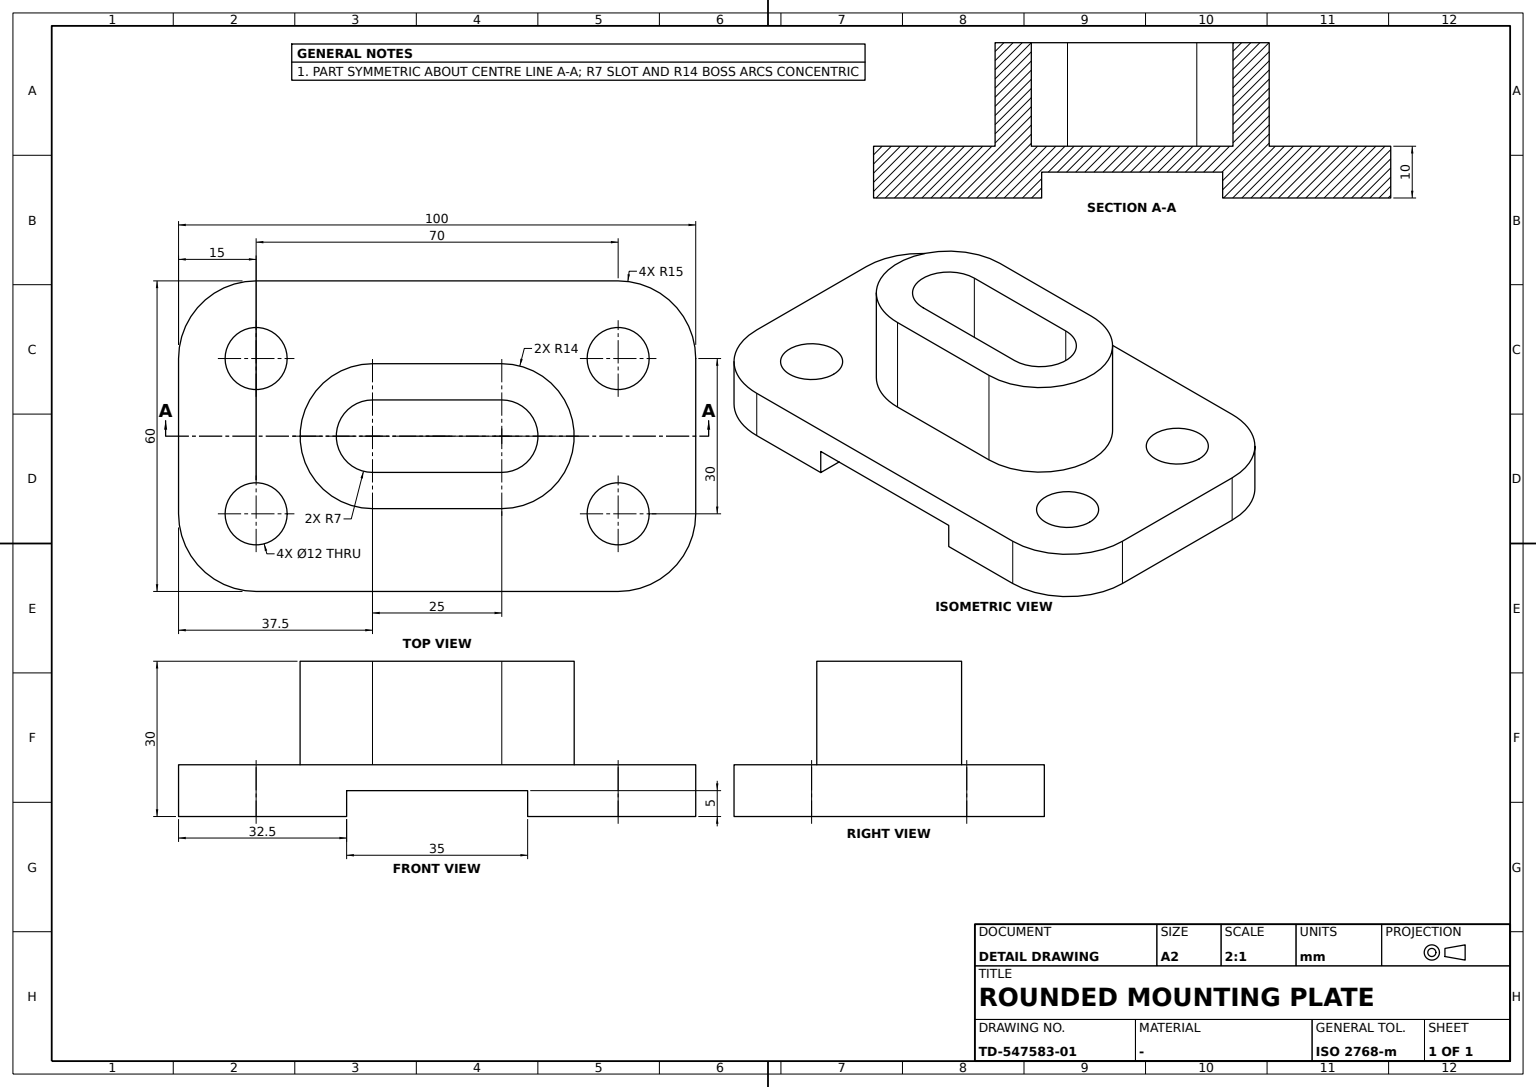
CATIA V5 part; units mm, degrees
sketch "Sketch1" plane through (0, 0, 0) normal (0, 0, 1) x (1, 0, 0)
  line L0 (50, 15) -> (50, -15)
  line L1 (35, -30) -> (-35, -30)
  line L2 (-50, -15) -> (-50, 15)
  line L3 (-35, 30) -> (35, 30)
  circle A0 centre (35, 15) radius 6
  circle A1 centre (-35, 15) radius 6
  circle A2 centre (-35, -15) radius 6
  circle A3 centre (35, -15) radius 6
  arc A4 (50, 15) -> (35, 30) centre (35, 15) ccw
  arc A5 (50, -15) -> (35, -30) centre (35, -15) cw
  arc A6 (-50, 15) -> (-35, 30) centre (-35, 15) cw
  arc A7 (-50, -15) -> (-35, -30) centre (-35, -15) ccw
  dimension "distance L1 L3" = 60
  dimension "distance L0 L2" = 100
  dimension "radius A0" = 6
  constraint vertical L0 y-axis
  constraint vertical L2 y-axis
  constraint horizontal L1 x-axis
  constraint horizontal L3 x-axis
  constraint equidistance L0 L2 origin
  constraint equidistance L1 L3 origin
  constraint symmetry A1 A2 x-axis
  constraint symmetry A0 A3 x-axis
  constraint symmetry A4 A5 x-axis
  constraint symmetry A4 A6 y-axis
  constraint symmetry A5 A7 y-axis
  constraint tangency A4 L3
extrude "Pad1" add sketch "Sketch1" along normal blind 10
sketch "Sketch2" plane through (0, 0, 10) normal (0, 0, 1) x (1, 0, 0)
  arc A0 (12.5, -7) -> (12.5, 7) centre (12.5, 0) ccw
  arc A1 (-12.5, -7) -> (-12.5, 7) centre (-12.5, 0) cw
  line L0 (-12.5, 14) -> (12.5, 14)
  line L1 (-12.5, -14) -> (12.5, -14)
  line L2 (-12.5, 7) -> (12.5, 7)
  line L3 (-12.5, -7) -> (12.5, -7)
  arc A2 (-12.5, -14) -> (-12.5, 14) centre (-12.5, 0) cw
  arc A3 (12.5, -14) -> (12.5, 14) centre (12.5, 0) ccw
  dimension "radius A0" = 7
  constraint symmetry A0 A1 y-axis
  constraint tangency L2 A1
  constraint tangency L2 A0
  constraint tangency L3 A1
  constraint tangency L3 A0
extrude "Pad2" add sketch "Sketch2" along normal blind 20
sketch "Sketch3" plane through (0, 30, 0) normal (0, 1, 0) x (-1, 0, 0)
  line L0 (17.5, 0) -> (17.5, 5)
  line L1 (17.5, 5) -> (-17.5, 5)
  line L2 (-17.5, 5) -> (-17.5, 0)
  line L3 (-17.5, 0) -> (17.5, 0)
  dimension "length L1" = 35
  constraint vertical L0 y-axis
  constraint vertical L2 y-axis
  constraint horizontal L1 x-axis
  constraint horizontal L3 x-axis
extrude "Pocket1" cut sketch "Sketch3" against normal through all
